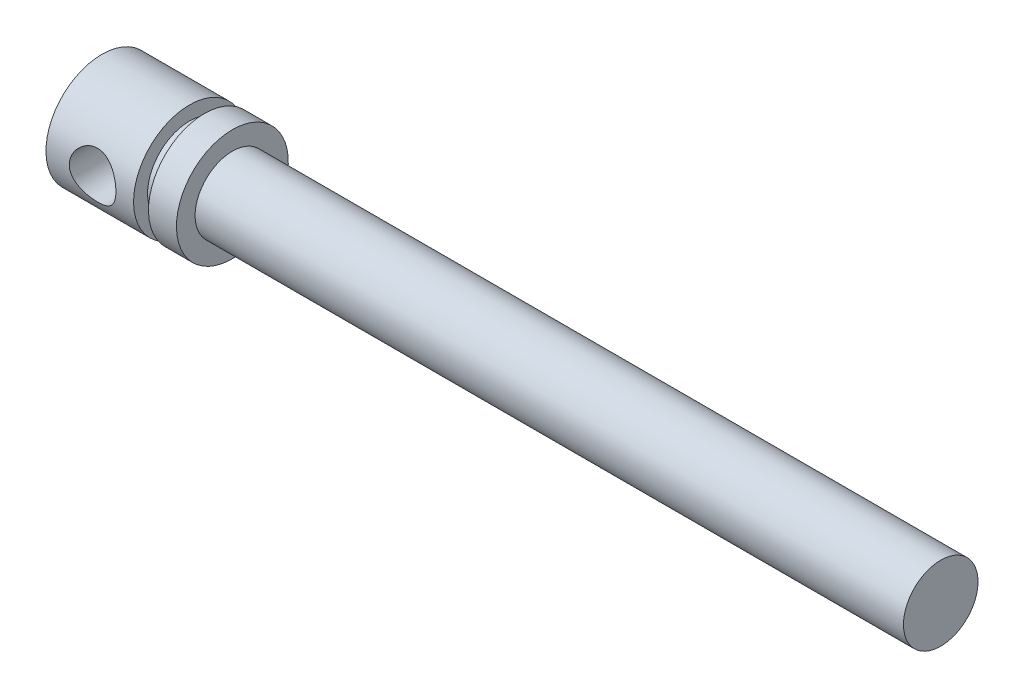
from build123d import *

# Parameters (mm, degrees)
CROSS_HOLE_DEPTH      = 91.39911504
CROSS_HOLE_DEPTH_BACK = 91.39911504
CROSS_HOLE_SKETCH_R   = 2.5


with BuildPart() as part:
    # Screw Profile Sketch → Screw Body Revolve (revolve)
    with BuildSketch(Plane.XY):
        Polygon((0, 0), (0, 6), (9.4, 6), (9.4, 4.5), (11, 4.5), (11, 6), (14, 6), (14, 4), (90, 4), (90, 0), align=None)
    revolve(axis=Axis((90, 0, 0), (-1, 0, 0)))

    # Cross Hole Sketch → Cross Hole (cut, two sides: drawn at the far end of the back side and taken through both)
    with BuildSketch(Plane.XY.offset(-CROSS_HOLE_DEPTH_BACK)):
        with Locations((5, 0)):
            Circle(CROSS_HOLE_SKETCH_R)
    extrude(amount=CROSS_HOLE_DEPTH + CROSS_HOLE_DEPTH_BACK, mode=Mode.SUBTRACT)


solid = part.part
